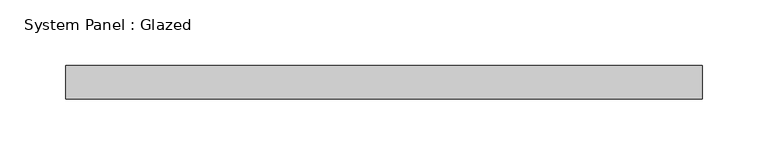
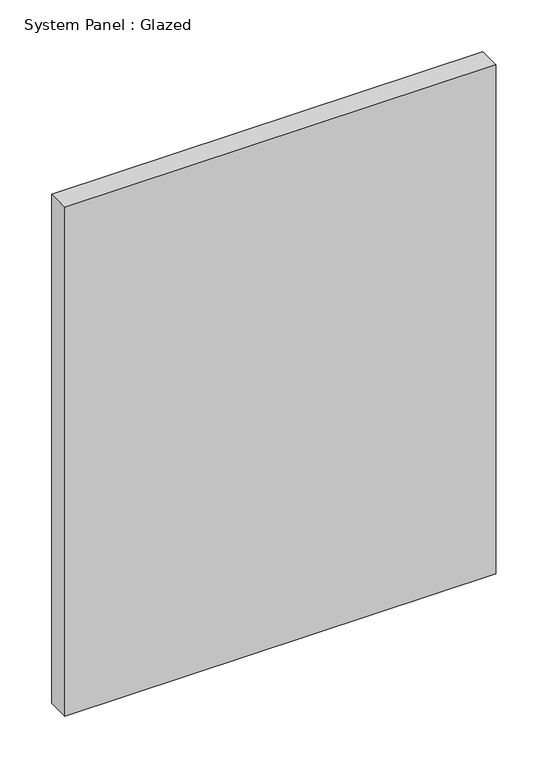
"""IFC4 building model written with IfcOpenShell, lengths in millimetres: plate geometry, System Panel : Glazed."""

from ifc_helpers import new_model, si_unit, origin, origin_with_axes, place, context, project, spatial, polyline, outline, extrude, source, transform, mapped, element, save


def system_panel_glazed_fe1d3f05(model_context):
    return source(origin(), model_context, "Body", "SweptSolid", [
        extrude(outline(polyline([(241.3, 19.05), (-241.3, 19.05), (-241.3, 44.45), (241.3, 44.45), (241.3, 19.05)])), origin_with_axes(), (0.0, 0.0, 1.0), 602.2276209),
    ])


if __name__ == "__main__":
    model = new_model("IFC4")
    model_context = context("Model", 3, world=origin())
    ifc_project = project(units=[si_unit("LENGTHUNIT", "METRE", prefix="MILLI")], contexts=[model_context])
    site = spatial("IfcSite", under=ifc_project)
    building = spatial("IfcBuilding", under=site)
    placement = place(None, origin())
    system_panel_glazed_shape = system_panel_glazed_fe1d3f05(model_context)
    element("IfcPlate", 1, ObjectType="System Panel : Glazed", at=placement, inside=building, context=model_context, shape_type="MappedRepresentation", body=[
        mapped(system_panel_glazed_shape, transform((0.0, 0.0, 0.0), x_axis=(1.0, 0.0, 0.0), y_axis=(0.0, 1.0, 0.0), z_axis=(0.0, 0.0, 1.0))),
    ])
    save(model, "model.ifc")

# Revit data of these elements
# Type "System Panel : Glazed"
#   Construction Type Id = "GSP4R"
#   Analytic Construction = "1/8 in Pilkington single glazing"
#   Visual Light Transmittance = 0.9
#   Solar Heat Gain Coefficient = 0.86
#   Heat Transfer Coefficient (U) = 1.18115 BTU/(h·ft²·°F)
#   Define Thermal Properties by = 1
# Element 1 (IfcPlate, "System Panel : Glazed")
#   Materials on its faces: "Glass"
# Materials
#   "Glass": class "Glass", colour RGB 0 128 192, transparency 0.75, Description = "Soda Lime Glass", Cost = 0
